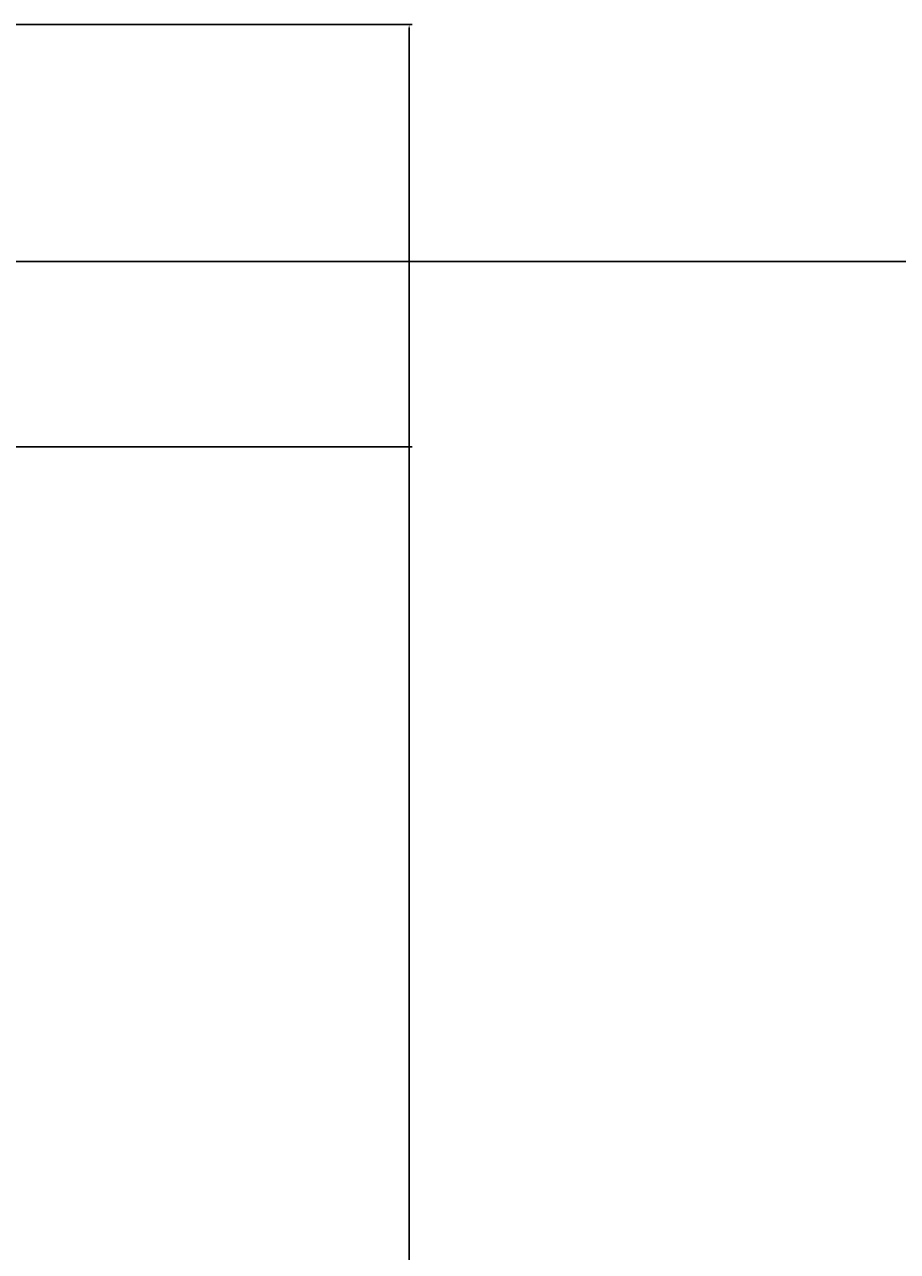
# Model space of a CAD drawing. Units: inches. Extents: x -128 to 854, y -395 to 398.
# Tile 57 of 61: x 368 to 417, y -248 to -178. Entities that reach past the tile are written whole.
import ezdxf

# ---------------------------------------------------------------- set-up
doc = ezdxf.new("R2010")
doc.units = ezdxf.units.IN
doc.header["$MEASUREMENT"] = 0
doc.layers.add('A-ANNO-DIMS', color=2, linetype='Continuous', lineweight=18)
doc.styles.get("Standard").update_dxf_attribs({"font": 'arial.ttf'})
doc.dimstyles.get("Standard").update_dxf_attribs({"dimtxt": 0.18, "dimasz": 0.18, "dimexe": 0.18, "dimexo": 0.0625, "dimgap": 0.09, "dimtad": 0, "dimtih": 1, "dimtoh": 1, "dimdec": 1, "dimzin": 0, "dimdsep": 46, "dimlunit": 4, "dimtxsty": 'Standard', "dimcen": 0.09, "dimclrd": 1, "dimclre": 2, "dimclrt": 6, "dimadec": 0, "dimazin": 0, "dimtfac": 1, "dimtdec": 1, "dimtofl": 0, "dimtmove": 0, "dimatfit": 3, "dimfxl": 1, "dimtfill": 2, "dimtfillclr": 3, "dimtolj": 1, "dimtzin": 0, "dimarcsym": 0})

# ---------------------------------------------------------------- blocks, each defined once
blk = doc.blocks.new('*D120')
at = {"layer": 'A-ANNO-DIMS', "color": 2, "lineweight": -2, "transparency": 16777216}
for p, q in [((317.902, -178.019), (389.719, -178.019)), ((337.902, -358.019), (389.719, -358.019))]:
    blk.add_line(p, q, dxfattribs=at)
at = {"layer": 'A-ANNO-DIMS', "color": 1, "lineweight": -2, "transparency": 16777216}
for p, q in [((389.539, -178.199), (389.539, -267.837)), ((389.539, -357.839), (389.539, -268.201))]:
    blk.add_line(p, q, dxfattribs=at)
at = {"layer": 'A-ANNO-DIMS', "color": 1, "transparency": 16777216}
for points in [[(389.509, -178.199), (389.569, -178.199), (389.539, -178.019)], [(389.509, -357.839), (389.569, -357.839), (389.539, -358.019)]]:
    blk.add_solid(points, dxfattribs=at)
at = {"layer": 'Defpoints', "color": 0, "transparency": 16777216}
for p in [(317.839, -178.019), (337.839, -358.019), (389.539, -358.019)]:
    blk.add_point(p, dxfattribs=at)
at = {"layer": 'A-ANNO-DIMS', "color": 6, "transparency": 16777216, "insert": (389.539, -268.019), "char_height": 0.18, "attachment_point": 5, "bg_fill": 1, "box_fill_scale": 1.25, "bg_fill_color": 3, "bg_fill_transparency": 0}
blk.add_mtext('\\A1;15\'-0"', dxfattribs=at)
blk = doc.blocks.new('*D127')
at = {"layer": 'A-ANNO-DIMS', "color": 2, "lineweight": -2, "transparency": 16777216}
for p, q in [((260.902, -202.019), (389.719, -202.019)), ((317.902, -298.019), (389.719, -298.019))]:
    blk.add_line(p, q, dxfattribs=at)
at = {"layer": 'A-ANNO-DIMS', "color": 1, "lineweight": -2, "transparency": 16777216}
for p, q in [((389.539, -202.199), (389.539, -249.837)), ((389.539, -297.839), (389.539, -250.201))]:
    blk.add_line(p, q, dxfattribs=at)
at = {"layer": 'A-ANNO-DIMS', "color": 1, "transparency": 16777216}
for points in [[(389.509, -202.199), (389.569, -202.199), (389.539, -202.019)], [(389.509, -297.839), (389.569, -297.839), (389.539, -298.019)]]:
    blk.add_solid(points, dxfattribs=at)
at = {"layer": 'Defpoints', "color": 0, "transparency": 16777216}
for p in [(260.839, -202.019), (389.539, -202.019), (317.839, -298.019)]:
    blk.add_point(p, dxfattribs=at)
at = {"layer": 'A-ANNO-DIMS', "color": 6, "transparency": 16777216, "insert": (389.539, -250.019), "char_height": 0.18, "attachment_point": 5, "bg_fill": 1, "box_fill_scale": 1.25, "bg_fill_color": 3, "bg_fill_transparency": 0}
blk.add_mtext('\\A1;8\'-0"', dxfattribs=at)
blk = doc.blocks.new('*D134')
at = {"layer": 'A-ANNO-DIMS', "color": 2, "lineweight": -2, "transparency": 16777216}
for p, q in [((418.217, -191.476), (346.3, -191.476)), ((418.217, -371.476), (346.3, -371.476))]:
    blk.add_line(p, q, dxfattribs=at)
at = {"layer": 'A-ANNO-DIMS', "color": 1, "lineweight": -2, "transparency": 16777216}
for p, q in [((346.48, -191.656), (346.48, -281.295)), ((346.48, -371.296), (346.48, -281.658))]:
    blk.add_line(p, q, dxfattribs=at)
at = {"layer": 'A-ANNO-DIMS', "color": 1, "transparency": 16777216}
for points in [[(346.45, -191.656), (346.51, -191.656), (346.48, -191.476)], [(346.45, -371.296), (346.51, -371.296), (346.48, -371.476)]]:
    blk.add_solid(points, dxfattribs=at)
at = {"layer": 'Defpoints', "color": 0, "transparency": 16777216}
for p in [(346.48, -191.476), (418.28, -191.476), (418.28, -371.476)]:
    blk.add_point(p, dxfattribs=at)
at = {"layer": 'A-ANNO-DIMS', "color": 6, "transparency": 16777216, "insert": (346.48, -281.476), "char_height": 0.18, "attachment_point": 5, "bg_fill": 1, "box_fill_scale": 1.25, "bg_fill_color": 3, "bg_fill_transparency": 0}
blk.add_mtext('\\A1;15\'-0"', dxfattribs=at)

msp = doc.modelspace()

# ---------------------------------------------------------------- dimensions: what is measured, and where the dimension line sits
at = {"layer": 'A-ANNO-DIMS'}
for base, p1, p2, picture, middle in [((389.539, -358.019), (317.839, -178.019), (337.839, -358.019), '*D120', (389.539, -268.019)), ((346.48, -191.476), (418.28, -371.476), (418.28, -191.476), '*D134', (346.48, -281.476)), ((389.539, -202.019), (317.839, -298.019), (260.839, -202.019), '*D127', (389.539, -250.019))]:
    dim = msp.add_linear_dim(base=base, p1=p1, p2=p2, angle=90, dimstyle='Standard', override={"dimdec": 1, "dimlfac": 1, "dimrnd": 0, "dimzin": 1, "dimdsep": 46, "dimlunit": 4, "dimfrac": 2}, dxfattribs=at)
    dim.commit()
    dim.dimension.update_dxf_attribs({"geometry": picture, "text_midpoint": middle})

doc.saveas('drawing.dxf')
